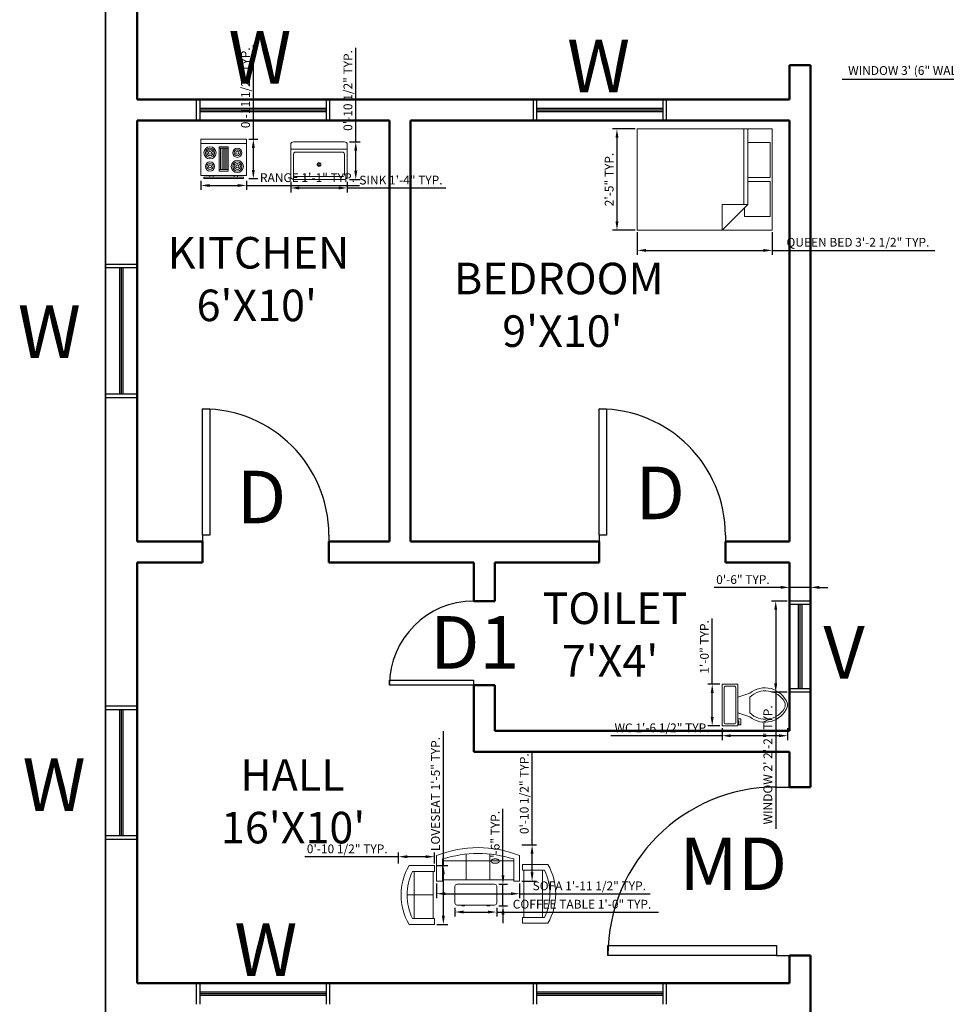
# Model space of a CAD drawing. Units: inches. Extents: x -25308 to -23933, y 10755 to 11996.
# Tile 2 of 6: x -25306 to -25042, y 11402 to 11683. Entities that reach past the tile are written whole.
import ezdxf

# ---------------------------------------------------------------- set-up
doc = ezdxf.new("R2010")
doc.units = ezdxf.units.IN
for name, color, linetype, lineweight in [('A-ANNO-DIMS', 2, 'Continuous', 18), ('A-ANNO-SYMB', 3, 'Continuous', 18), ('A-AREA-IDEN', 7, 'Continuous', 18), ('A-DOOR', 3, 'Continuous', 25), ('A-FLOR-FIXT', 8, 'Continuous', 18), ('A-FURN', 8, 'Continuous', 18), ('A-GLAZ', 4, 'Continuous', 25), ('A-WALL', 7, 'Continuous', 50), ('C-PROP', 30, 'Continuous', 35)]:
    doc.layers.add(name, color=color, linetype=linetype, lineweight=lineweight)
doc.styles.get("Standard").update_dxf_attribs({"font": 'arial.ttf'})
doc.dimstyles.new('ISO-25', dxfattribs={"dimtxt": 2.5, "dimasz": 2.5, "dimexe": 1.25, "dimexo": 0.625, "dimtad": 1, "dimdec": 0, "dimlunit": 3, "dimtxsty": 'Standard', "dimcen": 2.5, "dimadec": 0, "dimazin": 0, "dimtfac": 1, "dimtdec": 0, "dimtmove": 0, "dimatfit": 3, "dimfxl": 1, "dimarcsym": 0})

# ---------------------------------------------------------------- blocks, each defined once
blk = doc.blocks.new('*U8')
for p, q in [((0, 0), (0, -100)), ((750, 0), (750, -100))]:
    blk.add_line(p, q)
blk.add_lwpolyline([(0, 0), (0, 750), (43.75, 750), (43.75, 0)], close=True)
blk.add_arc((0, 0), 750, 0, 90)
blk = doc.blocks.new('Bed - Queen')
for p, q in [((0, -80.00003), (0, 0)), ((0, 0), (59.99999, 0)), ((59.99999, 0), (59.99999, -80.00003)), ((7.99999, -1.2), (28.79998, -1.2)), ((7.99999, -14.4), (7.99999, -1.2)), ((28.79998, -1.2), (28.79998, -14.4)), ((31.19999, -1.2), (51.99999, -1.2)), ((31.19999, -14.4), (31.19999, -1.2)), ((51.99999, -1.2), (51.99999, -16.4)), ((0, -14.4), (44.8, -14.4)), ((44.8, -16.8), (0, -16.8)), ((59.99999, -29.6), (44.8, -14.4)), ((44.8, -14.4), (44.8, -29.6)), ((51.99999, -16.4), (46.79936, -16.4)), ((44.8, -29.6), (59.99999, -29.6)), ((59.99999, -80.00003), (0, -80.00003))]:
    blk.add_line(p, q)
blk = doc.blocks.new('Range-Oven - 30 in top')
for p, q in [((0, -3), (30, -3)), ((12, -6), (18, -6)), ((13, -20), (13, -6)), ((14, -6), (14, -20)), ((15, -20), (15, -6)), ((16, -6), (16, -20)), ((17, -20), (17, -6)), ((6, -24), (6, -25)), ((8, -25), (8, -24)), ((18, -20), (12, -20)), ((22, -25), (22, -24)), ((24, -24), (24, -25))]:
    blk.add_line(p, q)
for points in [[(0, -24), (0, 0), (30, 0), (30, -24)], [(12, -21), (12, -5), (18, -5), (18, -21)], [(2, -26), (2, -25), (28, -25), (28, -26)]]:
    blk.add_lwpolyline(points, close=True)
for centre, radius in [((6, -9), 4), ((6, -9), 3), ((24, -9), 3), ((6, -9), 2), ((6, -9), 1), ((24, -9), 2), ((24, -9), 1), ((6, -18), 3), ((6, -18), 2), ((6, -18), 1), ((24, -18), 4), ((24, -18), 3), ((24, -18), 2), ((24, -18), 1)]:
    blk.add_circle(centre, radius)
blk = doc.blocks.new('Sink-single - 30 in top')
blk.add_line((-15, -3.999996), (15, -3.999996))
for points in [[(-13.5, 0), (13.5, 0)], [(-15, -18.499996), (-15, -1.5)], [(15, -1.5), (15, -18.499996)], [(-13.5, -17.499996), (-13.5, -6.499996)], [(-12.5, -5.499996), (12.5, -5.499996)], [(13.5, -6.499996), (13.5, -17.499996)], [(13.5, -19.999996), (-13.5, -19.999996)], [(12.5, -18.499996), (-12.5, -18.499996)]]:
    blk.add_lwpolyline(points)
for radius in [1, 0.5]:
    blk.add_circle((0, -11.999996), radius)
for centre, radius, start, end in [((-13.5, -1.5), 1.5, 90, 180), ((13.5, -1.5), 1.5, 0, 90), ((-12.5, -6.499996), 1, 90, 180), ((12.5, -6.499996), 1, 0, 90), ((-13.5, -18.499996), 1.5, 180, 270), ((-12.5, -17.499996), 1, 180, 270), ((12.5, -17.499996), 1, 270, 0), ((13.5, -18.499996), 1.5, 270, 0)]:
    blk.add_arc(centre, radius, start, end)
blk = doc.blocks.new('Toilet - top')
for p, q in [((9.5, -6), (9.5, -2)), ((-10, -8.5), (-8, -8.5)), ((-10, -9.5), (-10, -8.5)), ((-7, -9.5), (-10, -9.5)), ((-8, -8.5), (-8, -8)), ((-7, -8), (-7, -9.5)), ((-4, -8), (-6, -14)), ((4, -8), (6, -14)), ((4, -14), (-4, -14))]:
    blk.add_line(p, q)
blk.add_lwpolyline([(10.5, -8), (10.5, 0), (-10.5, 0), (-10.5, -8)], close=True)
for points in [[(-9.5, -2), (-9.5, -6)], [(8.5, -1), (-8.5, -1)], [(-8.5, -7), (8.5, -7)]]:
    blk.add_lwpolyline(points)
for centre, radius, start, end in [((-8.62, -1.88), 0.884, 81.8699, 188.1301), ((8.62, -1.88), 0.884, 351.8699, 98.1301), ((-8.62, -6.12), 0.884, 171.8699, 278.1301), ((8.62, -6.12), 0.884, 261.8699, 8.1301), ((3.52, -21.58), 12.17, 141.4691, 247.9714), ((4.2, -21.82), 11.33, 136.3677, 238.9468), ((-3.52, -21.58), 12.17, 292.0284, 38.5307), ((-4.2, -21.82), 11.33, 301.053, 43.6321), ((0, -27.88), 4, 245.7318, 294.2682), ((0, -29), 4, 254.8605, 285.1395)]:
    blk.add_arc(centre, radius, start, end)
blk = doc.blocks.new('Desk - 30 x 60 in.')
for p, q in [((-26.999995, 0), (26.999995, 0)), ((-29.999995, -27), (-29.999995, -3)), ((29.999995, -3), (29.999995, -27)), ((26.999995, -30), (-26.999995, -30)), ((-20.000005, -30), (-20.000005, -31)), ((-20.000005, -31), (-16.000005, -31)), ((-16.000005, -31), (-16.000005, -30)), ((15.999995, -31), (15.999995, -30)), ((19.999995, -31), (15.999995, -31)), ((19.999995, -30), (19.999995, -31))]:
    blk.add_line(p, q)
for centre, start, end in [((-26.499995, -3.5), 98.1301, 171.8699), ((26.499995, -3.5), 8.130102, 81.8699), ((-26.499995, -26.5), 188.1301, 261.8699), ((26.499995, -26.5), 278.1301, 351.8699)]:
    blk.add_arc(centre, 3.535534, start, end)
blk = doc.blocks.new('Sofa - Roundback 7 ft.')
for p, q in [((-12.00002, -32.4421), (-12.00003, -6.5971)), ((11.99997, -32.4421), (11.99998, -6.5971)), ((-36.000027, -34), (-36.000027, -11.4696)), ((-35.999844, -13.3819), (35.9998, -13.3819)), ((35.99998, -34), (35.99998, -11.4696)), ((-36.000027, -32.4421), (35.99998, -32.4421))]:
    blk.add_line(p, q)
for points in [[(-36.000027, -34), (-42.000027, -34), (-42.000027, -8)], [(41.99998, -8), (41.99998, -34), (35.99998, -34)]]:
    blk.add_lwpolyline(points)
for centre, radius, start, end in [((0, -114.25), 114.25, 68.43141, 111.5686), ((-0.00001, -127.1968), 121.1968, 72.72033, 107.2797)]:
    blk.add_arc(centre, radius, start, end)
blk = doc.blocks.new('Sofa - Roundback Loveseat 5 ft.')
for p, q in [((0, -32.44198), (0, -5.99998)), ((-24, -33.99998), (-24, -11.46958)), ((-23.9998, -13.38178), (23.99986, -13.38178)), ((24.00004, -33.99998), (24.00004, -11.46958)), ((-24, -32.44198), (24.00004, -32.44198))]:
    blk.add_line(p, q)
for points in [[(-24, -33.99998), (-30, -33.99998), (-30, -7.99998)], [(30.00004, -7.99998), (30.00004, -33.99998), (24.00004, -33.99998)]]:
    blk.add_lwpolyline(points)
for centre, radius, start, end in [((0, -60.24998), 60.24998, 60.13715, 119.8628), ((0, -61.38438), 55.38444, 64.32083, 115.6792)]:
    blk.add_arc(centre, radius, start, end)
blk = doc.blocks.new('WIN-36-9IN')
for p, q in [((0, 9), (0, 0)), ((1, 9), (1, 0)), ((37, 9), (37, 0)), ((38, 9), (38, 0)), ((1, 5), (37, 5)), ((1, 4.5), (37, 4.5)), ((1, 4), (37, 4))]:
    blk.add_line(p, q)
blk = doc.blocks.new('WIN-24-6IN')
for p, q in [((0, 26), (6, 26)), ((0, 25), (6, 25)), ((2.5, 1), (2.5, 25)), ((3, 1), (3, 25)), ((3.5, 1), (3.5, 25)), ((0, 1), (6, 1)), ((0, 0), (6, 0))]:
    blk.add_line(p, q)
blk = doc.blocks.new('WIN-36-6IN')
for p, q in [((0, 6), (0, 0)), ((1, 6), (1, 0)), ((37, 6), (37, 0)), ((38, 6), (38, 0)), ((1, 3.5), (37, 3.5)), ((1, 3), (37, 3)), ((1, 2.5), (37, 2.5))]:
    blk.add_line(p, q)
blk = doc.blocks.new('*D184')
at = {"layer": 'A-ANNO-DIMS', "color": 0, "lineweight": -2, "transparency": 16777216}
for p, q in [((-25015.44, 11660.75), (-25015.44, 11667.07)), ((-24977.44, 11660.75), (-24977.44, 11667.07)), ((-25015.44, 11665.82), (-25071.37, 11665.82)), ((-24979.94, 11665.82), (-25012.94, 11665.82))]:
    blk.add_line(p, q, dxfattribs=at)
at = {"layer": 'A-ANNO-DIMS', "color": 0, "transparency": 16777216}
for points in [[(-25012.94, 11666.24), (-25012.94, 11665.4), (-25015.44, 11665.82)], [(-24979.94, 11666.24), (-24979.94, 11665.4), (-24977.44, 11665.82)]]:
    blk.add_solid(points, dxfattribs=at)
at = {"layer": 'Defpoints', "color": 0, "transparency": 16777216}
for p in [(-25015.44, 11665.82), (-25015.44, 11660.12), (-24977.44, 11660.12)]:
    blk.add_point(p, dxfattribs=at)
at = {"layer": 'A-ANNO-DIMS', "color": 0, "transparency": 16777216, "insert": (-25044.66, 11668.09), "char_height": 2.5, "attachment_point": 5}
blk.add_mtext('WINDOW 3\' (6" WALL) 3\'-2" TYP.', dxfattribs=at)
blk = doc.blocks.new('*D186')
at = {"layer": 'A-ANNO-DIMS', "color": 0, "lineweight": -2, "transparency": 16777216}
for p, q in [((-25087.07, 11517.12), (-25091.59, 11517.12)), ((-25090.34, 11514.62), (-25090.34, 11493.62)), ((-25087.07, 11491.12), (-25091.59, 11491.12)), ((-25090.34, 11491.12), (-25090.34, 11452.16))]:
    blk.add_line(p, q, dxfattribs=at)
at = {"layer": 'A-ANNO-DIMS', "color": 0, "transparency": 16777216}
for points in [[(-25090.76, 11514.62), (-25089.93, 11514.62), (-25090.34, 11517.12)], [(-25090.76, 11493.62), (-25089.93, 11493.62), (-25090.34, 11491.12)]]:
    blk.add_solid(points, dxfattribs=at)
at = {"layer": 'Defpoints', "color": 0, "transparency": 16777216}
for p in [(-25086.44, 11517.12), (-25090.34, 11491.12), (-25086.44, 11491.12)]:
    blk.add_point(p, dxfattribs=at)
at = {"layer": 'A-ANNO-DIMS', "color": 0, "transparency": 16777216, "insert": (-25092.26, 11470.39), "char_height": 2.5, "attachment_point": 5, "rotation": 90}
blk.add_mtext('WINDOW 2\' 2\'-2" TYP.', dxfattribs=at)
blk = doc.blocks.new('*D187')
at = {"layer": 'A-ANNO-DIMS', "color": 0, "lineweight": -2, "transparency": 16777216}
for p, q in [((-25088.94, 11521.02), (-25107.93, 11521.02)), ((-25086.44, 11517.75), (-25086.44, 11522.27)), ((-25080.44, 11521.02), (-25086.44, 11521.02)), ((-25080.44, 11517.75), (-25080.44, 11522.27)), ((-25077.94, 11521.02), (-25075.44, 11521.02))]:
    blk.add_line(p, q, dxfattribs=at)
at = {"layer": 'A-ANNO-DIMS', "color": 0, "transparency": 16777216}
for points in [[(-25088.94, 11521.44), (-25088.94, 11520.6), (-25086.44, 11521.02)], [(-25077.94, 11521.44), (-25077.94, 11520.6), (-25080.44, 11521.02)]]:
    blk.add_solid(points, dxfattribs=at)
at = {"layer": 'Defpoints', "color": 0, "transparency": 16777216}
for p in [(-25086.44, 11521.02), (-25086.44, 11517.12), (-25080.44, 11517.12)]:
    blk.add_point(p, dxfattribs=at)
at = {"layer": 'A-ANNO-DIMS', "color": 0, "transparency": 16777216, "insert": (-25099.69, 11522.92), "char_height": 2.5, "attachment_point": 5}
blk.add_mtext('0\'-6" TYP.', dxfattribs=at)
blk = doc.blocks.new('*D192')
at = {"layer": 'A-ANNO-DIMS', "color": 0, "lineweight": -2, "transparency": 16777216}
for p, q in [((-25185.1, 11441.7), (-25185.1, 11479.98)), ((-25187, 11441.7), (-25183.85, 11441.7)), ((-25185.1, 11427.41), (-25185.1, 11439.2)), ((-25187, 11424.91), (-25183.85, 11424.91))]:
    blk.add_line(p, q, dxfattribs=at)
at = {"layer": 'A-ANNO-DIMS', "color": 0, "transparency": 16777216}
for points in [[(-25185.52, 11439.2), (-25184.68, 11439.2), (-25185.1, 11441.7)], [(-25185.52, 11427.41), (-25184.68, 11427.41), (-25185.1, 11424.91)]]:
    blk.add_solid(points, dxfattribs=at)
at = {"layer": 'Defpoints', "color": 0, "transparency": 16777216}
for p in [(-25187.62, 11441.7), (-25185.1, 11441.7), (-25187.62, 11424.91)]:
    blk.add_point(p, dxfattribs=at)
at = {"layer": 'A-ANNO-DIMS', "color": 0, "transparency": 16777216, "insert": (-25187.02, 11462.09), "char_height": 2.5, "attachment_point": 5, "rotation": 90}
blk.add_mtext('LOVESEAT 1\'-5" TYP.', dxfattribs=at)
blk = doc.blocks.new('*D193')
at = {"layer": 'A-ANNO-DIMS', "color": 0, "lineweight": -2, "transparency": 16777216}
for p, q in [((-25197.88, 11442.32), (-25197.88, 11445.46)), ((-25187.62, 11442.32), (-25187.62, 11445.46)), ((-25197.88, 11444.21), (-25224.64, 11444.21)), ((-25190.12, 11444.21), (-25195.38, 11444.21))]:
    blk.add_line(p, q, dxfattribs=at)
at = {"layer": 'A-ANNO-DIMS', "color": 0, "transparency": 16777216}
for points in [[(-25195.38, 11444.63), (-25195.38, 11443.8), (-25197.88, 11444.21)], [(-25190.12, 11444.63), (-25190.12, 11443.8), (-25187.62, 11444.21)]]:
    blk.add_solid(points, dxfattribs=at)
at = {"layer": 'Defpoints', "color": 0, "transparency": 16777216}
for p in [(-25197.88, 11444.21), (-25197.88, 11441.7), (-25187.62, 11441.7)]:
    blk.add_point(p, dxfattribs=at)
at = {"layer": 'A-ANNO-DIMS', "color": 0, "transparency": 16777216, "insert": (-25212.51, 11446.13), "char_height": 2.5, "attachment_point": 5}
blk.add_mtext('0\'-10 1/2" TYP.', dxfattribs=at)
blk = doc.blocks.new('*D198')
at = {"layer": 'A-ANNO-DIMS', "color": 0, "lineweight": -2, "transparency": 16777216}
for p, q in [((-25187.05, 11436.59), (-25187.05, 11432.41)), ((-25163.36, 11436.59), (-25163.36, 11432.41)), ((-25184.55, 11433.66), (-25165.86, 11433.66)), ((-25163.36, 11433.66), (-25126.13, 11433.66))]:
    blk.add_line(p, q, dxfattribs=at)
at = {"layer": 'A-ANNO-DIMS', "color": 0, "transparency": 16777216}
for points in [[(-25184.55, 11434.08), (-25184.55, 11433.24), (-25187.05, 11433.66)], [(-25165.86, 11434.08), (-25165.86, 11433.24), (-25163.36, 11433.66)]]:
    blk.add_solid(points, dxfattribs=at)
at = {"layer": 'Defpoints', "color": 0, "transparency": 16777216}
for p in [(-25187.05, 11437.21), (-25163.36, 11437.21), (-25163.36, 11433.66)]:
    blk.add_point(p, dxfattribs=at)
at = {"layer": 'A-ANNO-DIMS', "color": 0, "transparency": 16777216, "insert": (-25143.5, 11435.58), "char_height": 2.5, "attachment_point": 5}
blk.add_mtext('SOFA 1\'-11 1/2" TYP.', dxfattribs=at)
blk = doc.blocks.new('*D199')
at = {"layer": 'A-ANNO-DIMS', "color": 0, "lineweight": -2, "transparency": 16777216}
for p, q in [((-25159.81, 11447.56), (-25159.81, 11474.31)), ((-25162.73, 11447.56), (-25158.56, 11447.56)), ((-25159.81, 11439.71), (-25159.81, 11445.06)), ((-25162.73, 11437.21), (-25158.56, 11437.21))]:
    blk.add_line(p, q, dxfattribs=at)
at = {"layer": 'A-ANNO-DIMS', "color": 0, "transparency": 16777216}
for points in [[(-25160.22, 11445.06), (-25159.39, 11445.06), (-25159.81, 11447.56)], [(-25160.22, 11439.71), (-25159.39, 11439.71), (-25159.81, 11437.21)]]:
    blk.add_solid(points, dxfattribs=at)
at = {"layer": 'Defpoints', "color": 0, "transparency": 16777216}
for p in [(-25163.36, 11447.56), (-25159.81, 11447.56), (-25163.36, 11437.21)]:
    blk.add_point(p, dxfattribs=at)
at = {"layer": 'A-ANNO-DIMS', "color": 0, "transparency": 16777216, "insert": (-25161.72, 11462.18), "char_height": 2.5, "attachment_point": 5, "rotation": 90}
blk.add_mtext('0\'-10 1/2" TYP.', dxfattribs=at)
blk = doc.blocks.new('*D204')
at = {"layer": 'A-ANNO-DIMS', "color": 0, "lineweight": -2, "transparency": 16777216}
for p, q in [((-25181.83, 11429.6), (-25181.83, 11427.18)), ((-25179.33, 11428.43), (-25172.39, 11428.43)), ((-25169.89, 11429.6), (-25169.89, 11427.18)), ((-25169.89, 11428.43), (-25123.76, 11428.43))]:
    blk.add_line(p, q, dxfattribs=at)
at = {"layer": 'A-ANNO-DIMS', "color": 0, "transparency": 16777216}
for points in [[(-25179.33, 11428.85), (-25179.33, 11428.02), (-25181.83, 11428.43)], [(-25172.39, 11428.85), (-25172.39, 11428.02), (-25169.89, 11428.43)]]:
    blk.add_solid(points, dxfattribs=at)
at = {"layer": 'Defpoints', "color": 0, "transparency": 16777216}
for p in [(-25181.83, 11430.22), (-25169.89, 11430.22), (-25169.89, 11428.43)]:
    blk.add_point(p, dxfattribs=at)
at = {"layer": 'A-ANNO-DIMS', "color": 0, "transparency": 16777216, "insert": (-25145.57, 11430.35), "char_height": 2.5, "attachment_point": 5}
blk.add_mtext('COFFEE TABLE 1\'-0" TYP.', dxfattribs=at)
blk = doc.blocks.new('*D205')
at = {"layer": 'A-ANNO-DIMS', "color": 0, "lineweight": -2, "transparency": 16777216}
for p, q in [((-25168.1, 11438.89), (-25168.1, 11457.88)), ((-25169.26, 11436.39), (-25166.85, 11436.39)), ((-25168.1, 11430.22), (-25168.1, 11436.39)), ((-25169.26, 11430.22), (-25166.85, 11430.22)), ((-25168.1, 11427.72), (-25168.1, 11425.22))]:
    blk.add_line(p, q, dxfattribs=at)
at = {"layer": 'A-ANNO-DIMS', "color": 0, "transparency": 16777216}
for points in [[(-25168.51, 11438.89), (-25167.68, 11438.89), (-25168.1, 11436.39)], [(-25168.51, 11427.72), (-25167.68, 11427.72), (-25168.1, 11430.22)]]:
    blk.add_solid(points, dxfattribs=at)
at = {"layer": 'Defpoints', "color": 0, "transparency": 16777216}
for p in [(-25169.89, 11436.39), (-25168.1, 11436.39), (-25169.89, 11430.22)]:
    blk.add_point(p, dxfattribs=at)
at = {"layer": 'A-ANNO-DIMS', "color": 0, "transparency": 16777216, "insert": (-25170, 11449.64), "char_height": 2.5, "attachment_point": 5, "rotation": 90}
blk.add_mtext('0\'-6" TYP.', dxfattribs=at)
blk = doc.blocks.new('*D206')
at = {"layer": 'A-ANNO-DIMS', "color": 0, "lineweight": -2, "transparency": 16777216}
for p, q in [((-25129.83, 11622.27), (-25129.83, 11615.87)), ((-25091.33, 11622.27), (-25091.33, 11615.87)), ((-25127.33, 11617.12), (-25093.83, 11617.12)), ((-25091.33, 11617.12), (-25044.98, 11617.12))]:
    blk.add_line(p, q, dxfattribs=at)
at = {"layer": 'A-ANNO-DIMS', "color": 0, "transparency": 16777216}
for points in [[(-25127.33, 11617.53), (-25127.33, 11616.7), (-25129.83, 11617.12)], [(-25093.83, 11617.53), (-25093.83, 11616.7), (-25091.33, 11617.12)]]:
    blk.add_solid(points, dxfattribs=at)
at = {"layer": 'Defpoints', "color": 0, "transparency": 16777216}
for p in [(-25129.83, 11622.89), (-25091.33, 11622.89), (-25091.33, 11617.12)]:
    blk.add_point(p, dxfattribs=at)
at = {"layer": 'A-ANNO-DIMS', "color": 0, "transparency": 16777216, "insert": (-25066.91, 11619.11), "char_height": 2.5, "attachment_point": 5}
blk.add_mtext('QUEEN BED 3\'-2 1/2" TYP.', dxfattribs=at)
blk = doc.blocks.new('*D207')
at = {"layer": 'A-ANNO-DIMS', "color": 0, "lineweight": -2, "transparency": 16777216}
for p, q in [((-25130.46, 11651.77), (-25136.86, 11651.77)), ((-25135.61, 11649.27), (-25135.61, 11625.39)), ((-25130.46, 11622.89), (-25136.86, 11622.89))]:
    blk.add_line(p, q, dxfattribs=at)
at = {"layer": 'A-ANNO-DIMS', "color": 0, "transparency": 16777216}
for points in [[(-25136.02, 11649.27), (-25135.19, 11649.27), (-25135.61, 11651.77)], [(-25136.02, 11625.39), (-25135.19, 11625.39), (-25135.61, 11622.89)]]:
    blk.add_solid(points, dxfattribs=at)
at = {"layer": 'Defpoints', "color": 0, "transparency": 16777216}
for p in [(-25129.83, 11651.77), (-25135.61, 11622.89), (-25129.83, 11622.89)]:
    blk.add_point(p, dxfattribs=at)
at = {"layer": 'A-ANNO-DIMS', "color": 0, "transparency": 16777216, "insert": (-25137.51, 11637.33), "char_height": 2.5, "attachment_point": 5, "rotation": 90}
blk.add_mtext('2\'-5" TYP.', dxfattribs=at)
blk = doc.blocks.new('*D210')
at = {"layer": 'A-ANNO-DIMS', "color": 0, "lineweight": -2, "transparency": 16777216}
for p, q in [((-25254.24, 11636.95), (-25254.24, 11634.38)), ((-25241.22, 11636.95), (-25241.22, 11634.38)), ((-25251.74, 11635.63), (-25243.72, 11635.63)), ((-25241.22, 11635.63), (-25208.97, 11635.63))]:
    blk.add_line(p, q, dxfattribs=at)
at = {"layer": 'A-ANNO-DIMS', "color": 0, "transparency": 16777216}
for points in [[(-25251.74, 11636.04), (-25251.74, 11635.21), (-25254.24, 11635.63)], [(-25243.72, 11636.04), (-25243.72, 11635.21), (-25241.22, 11635.63)]]:
    blk.add_solid(points, dxfattribs=at)
at = {"layer": 'Defpoints', "color": 0, "transparency": 16777216}
for p in [(-25254.24, 11637.58), (-25241.22, 11637.58), (-25241.22, 11635.63)]:
    blk.add_point(p, dxfattribs=at)
at = {"layer": 'A-ANNO-DIMS', "color": 0, "transparency": 16777216, "insert": (-25223.85, 11637.54), "char_height": 2.5, "attachment_point": 5}
blk.add_mtext('RANGE 1\'-1" TYP.', dxfattribs=at)
blk = doc.blocks.new('*D211')
at = {"layer": 'A-ANNO-DIMS', "color": 0, "lineweight": -2, "transparency": 16777216}
for p, q in [((-25239.27, 11648.86), (-25239.27, 11675.61)), ((-25240.6, 11648.86), (-25238.02, 11648.86)), ((-25239.27, 11640.08), (-25239.27, 11646.36)), ((-25240.6, 11637.58), (-25238.02, 11637.58))]:
    blk.add_line(p, q, dxfattribs=at)
at = {"layer": 'A-ANNO-DIMS', "color": 0, "transparency": 16777216}
for points in [[(-25239.69, 11646.36), (-25238.85, 11646.36), (-25239.27, 11648.86)], [(-25239.69, 11640.08), (-25238.85, 11640.08), (-25239.27, 11637.58)]]:
    blk.add_solid(points, dxfattribs=at)
at = {"layer": 'Defpoints', "color": 0, "transparency": 16777216}
for p in [(-25241.22, 11648.86), (-25239.27, 11648.86), (-25241.22, 11637.58)]:
    blk.add_point(p, dxfattribs=at)
at = {"layer": 'A-ANNO-DIMS', "color": 0, "transparency": 16777216, "insert": (-25241.19, 11663.49), "char_height": 2.5, "attachment_point": 5, "rotation": 90}
blk.add_mtext('0\'-11 1/2" TYP.', dxfattribs=at)
blk = doc.blocks.new('*D212')
at = {"layer": 'A-ANNO-DIMS', "color": 0, "lineweight": -2, "transparency": 16777216}
for p, q in [((-25105.65, 11478.72), (-25137.36, 11478.72)), ((-25105.65, 11480.9), (-25105.65, 11477.47)), ((-25089.45, 11478.72), (-25103.15, 11478.72)), ((-25086.95, 11480.9), (-25086.95, 11477.47))]:
    blk.add_line(p, q, dxfattribs=at)
at = {"layer": 'A-ANNO-DIMS', "color": 0, "transparency": 16777216}
for points in [[(-25103.15, 11479.14), (-25103.15, 11478.3), (-25105.65, 11478.72)], [(-25089.45, 11479.14), (-25089.45, 11478.3), (-25086.95, 11478.72)]]:
    blk.add_solid(points, dxfattribs=at)
at = {"layer": 'Defpoints', "color": 0, "transparency": 16777216}
for p in [(-25105.65, 11481.52), (-25086.95, 11481.52), (-25105.65, 11478.72)]:
    blk.add_point(p, dxfattribs=at)
at = {"layer": 'A-ANNO-DIMS', "color": 0, "transparency": 16777216, "insert": (-25122.76, 11480.64), "char_height": 2.5, "attachment_point": 5}
blk.add_mtext('WC 1\'-6 1/2" TYP.', dxfattribs=at)
blk = doc.blocks.new('*D213')
at = {"layer": 'A-ANNO-DIMS', "color": 0, "lineweight": -2, "transparency": 16777216}
for p, q in [((-25108.46, 11493.41), (-25108.46, 11512.16)), ((-25106.28, 11493.41), (-25109.71, 11493.41)), ((-25108.46, 11484.02), (-25108.46, 11490.91)), ((-25106.28, 11481.52), (-25109.71, 11481.52))]:
    blk.add_line(p, q, dxfattribs=at)
at = {"layer": 'A-ANNO-DIMS', "color": 0, "transparency": 16777216}
for points in [[(-25108.87, 11490.91), (-25108.04, 11490.91), (-25108.46, 11493.41)], [(-25108.87, 11484.02), (-25108.04, 11484.02), (-25108.46, 11481.52)]]:
    blk.add_solid(points, dxfattribs=at)
at = {"layer": 'Defpoints', "color": 0, "transparency": 16777216}
for p in [(-25108.46, 11493.41), (-25105.65, 11493.41), (-25105.65, 11481.52)]:
    blk.add_point(p, dxfattribs=at)
at = {"layer": 'A-ANNO-DIMS', "color": 0, "transparency": 16777216, "insert": (-25110.36, 11504.04), "char_height": 2.5, "attachment_point": 5, "rotation": 90}
blk.add_mtext('1\'-0" TYP.', dxfattribs=at)
blk = doc.blocks.new('*D216')
at = {"layer": 'A-ANNO-DIMS', "color": 0, "lineweight": -2, "transparency": 16777216}
for p, q in [((-25228.62, 11636.71), (-25228.62, 11633.67)), ((-25212.49, 11636.71), (-25212.49, 11633.67)), ((-25226.12, 11634.92), (-25214.99, 11634.92)), ((-25212.49, 11634.92), (-25184.4, 11634.92))]:
    blk.add_line(p, q, dxfattribs=at)
at = {"layer": 'A-ANNO-DIMS', "color": 0, "transparency": 16777216}
for points in [[(-25226.12, 11635.34), (-25226.12, 11634.5), (-25228.62, 11634.92)], [(-25214.99, 11635.34), (-25214.99, 11634.5), (-25212.49, 11634.92)]]:
    blk.add_solid(points, dxfattribs=at)
at = {"layer": 'Defpoints', "color": 0, "transparency": 16777216}
for p in [(-25228.62, 11637.34), (-25212.49, 11637.34), (-25212.49, 11634.92)]:
    blk.add_point(p, dxfattribs=at)
at = {"layer": 'A-ANNO-DIMS', "color": 0, "transparency": 16777216, "insert": (-25197.19, 11636.84), "char_height": 2.5, "attachment_point": 5}
blk.add_mtext('SINK 1\'-4" TYP.', dxfattribs=at)
blk = doc.blocks.new('*D217')
at = {"layer": 'A-ANNO-DIMS', "color": 0, "lineweight": -2, "transparency": 16777216}
for p, q in [((-25210.08, 11648.09), (-25210.08, 11674.84)), ((-25211.87, 11648.09), (-25208.83, 11648.09)), ((-25210.08, 11639.84), (-25210.08, 11645.59)), ((-25211.87, 11637.34), (-25208.83, 11637.34))]:
    blk.add_line(p, q, dxfattribs=at)
at = {"layer": 'A-ANNO-DIMS', "color": 0, "transparency": 16777216}
for points in [[(-25210.49, 11645.59), (-25209.66, 11645.59), (-25210.08, 11648.09)], [(-25210.49, 11639.84), (-25209.66, 11639.84), (-25210.08, 11637.34)]]:
    blk.add_solid(points, dxfattribs=at)
at = {"layer": 'Defpoints', "color": 0, "transparency": 16777216}
for p in [(-25212.49, 11648.09), (-25210.08, 11648.09), (-25212.49, 11637.34)]:
    blk.add_point(p, dxfattribs=at)
at = {"layer": 'A-ANNO-DIMS', "color": 0, "transparency": 16777216, "insert": (-25211.99, 11662.72), "char_height": 2.5, "attachment_point": 5, "rotation": 90}
blk.add_mtext('0\'-10 1/2" TYP.', dxfattribs=at)

msp = doc.modelspace()

# ---------------------------------------------------------------- linework, layer by layer
at = {"layer": 'A-WALL'}
for p, q in [((-25272.44, 11660.12), (-25272.44, 11780.12)), ((-25086.44, 11660.12), (-25086.44, 11669.94)), ((-25086.44, 11669.94), (-25080.44, 11669.94)), ((-25080.44, 11464.06), (-25080.44, 11669.94)), ((-25272.44, 11660.12), (-25086.44, 11660.12)), ((-25272.44, 11654.12), (-25200.44, 11654.12)), ((-25272.44, 11534.12), (-25272.44, 11654.12)), ((-25200.44, 11534.12), (-25200.44, 11654.12)), ((-25194.44, 11534.12), (-25194.44, 11654.12)), ((-25194.44, 11654.12), (-25086.44, 11654.12)), ((-25086.44, 11534.12), (-25086.44, 11654.12)), ((-25272.44, 11534.12), (-25253.74, 11534.12)), ((-25253.74, 11534.12), (-25253.74, 11528.12)), ((-25217.74, 11534.12), (-25217.74, 11528.12)), ((-25217.74, 11534.12), (-25200.44, 11534.12)), ((-25194.44, 11534.12), (-25140.68, 11534.12)), ((-25140.68, 11534.12), (-25140.68, 11528.12)), ((-25104.68, 11534.12), (-25104.68, 11528.12)), ((-25104.68, 11534.12), (-25086.44, 11534.12)), ((-25272.44, 11528.12), (-25253.74, 11528.12)), ((-25272.44, 11408.12), (-25272.44, 11528.12)), ((-25217.74, 11528.12), (-25176.44, 11528.12)), ((-25176.44, 11517.12), (-25176.44, 11528.12)), ((-25176.44, 11517.12), (-25176.44, 11528.12)), ((-25176.44, 11517.12), (-25176.44, 11528.12)), ((-25170.44, 11528.12), (-25140.68, 11528.12)), ((-25170.44, 11517.12), (-25170.44, 11528.12)), ((-25170.44, 11517.12), (-25170.44, 11528.12)), ((-25170.44, 11517.12), (-25170.44, 11528.12)), ((-25104.68, 11528.12), (-25086.44, 11528.12)), ((-25086.44, 11480.12), (-25086.44, 11528.12)), ((-25176.44, 11517.12), (-25170.44, 11517.12)), ((-25176.44, 11474.12), (-25176.44, 11493.12)), ((-25176.44, 11474.12), (-25176.44, 11493.12)), ((-25176.44, 11474.12), (-25176.44, 11493.12)), ((-25176.44, 11493.12), (-25170.44, 11493.12)), ((-25170.44, 11480.12), (-25170.44, 11493.12)), ((-25170.44, 11480.12), (-25170.44, 11493.12)), ((-25170.44, 11480.12), (-25170.44, 11493.12)), ((-25170.44, 11480.12), (-25086.44, 11480.12)), ((-25176.44, 11474.12), (-25086.44, 11474.12)), ((-25086.44, 11464.06), (-25086.44, 11474.12)), ((-25086.44, 11464.06), (-25080.44, 11464.06)), ((-25086.44, 11408.12), (-25086.44, 11416.06)), ((-25086.44, 11416.06), (-25080.44, 11416.06)), ((-25080.44, 11213.16), (-25080.44, 11416.06)), ((-25272.44, 11408.12), (-25086.44, 11408.12))]:
    msp.add_line(p, q, dxfattribs=at)
at = {"layer": 'C-PROP'}
msp.add_line((-25281.44, 10811.12), (-25281.44, 11915.12), dxfattribs=at)

# ---------------------------------------------------------------- block references
at = {"layer": 'A-DOOR', "xscale": 0.0480000000000013, "yscale": 0.0480000000000013, "zscale": 0.0480000000000013}
for p in [(-25253.74, 11535.92), (-25140.68, 11535.92)]:
    msp.add_blockref('*U8', p, dxfattribs=at)
at = {"layer": 'A-DOOR', "rotation": 90}
for p, xscale, yscale, zscale in [((-25176.47, 11493.12), 0.0320000000000009, 0.0320000000000009, 0.0320000000000009), ((-25090.14, 11416.06), 0.0640305237838995, 0.0640305237838995, 0.0640305237838995)]:
    msp.add_blockref('*U8', p, dxfattribs=dict(at, xscale=xscale, yscale=yscale, zscale=zscale))
at = {"layer": 'A-FLOR-FIXT'}
for name, p, xscale, yscale, zscale in [('Range-Oven - 30 in top', (-25254.24, 11648.86), 0.4338097128947254, 0.4338097128947254, 0.4338097128947254), ('Sink-single - 30 in top', (-25220.56, 11648.09), 0.5374838416175965, 0.5374838416175965, 0.5374838416175965)]:
    msp.add_blockref(name, p, dxfattribs=dict(at, xscale=xscale, yscale=yscale, zscale=zscale))
at = {"layer": 'A-FLOR-FIXT', "xscale": 0.5659332238665749, "yscale": 0.5659332238665749, "zscale": 0.5659332238665749, "rotation": 90}
msp.add_blockref('Toilet - top', (-25105.65, 11487.47), dxfattribs=at)
at = {"layer": 'A-FURN'}
for name, p, xscale, yscale, zscale, rotation in [('Bed - Queen', (-25091.33, 11651.77), 0.4812808282186369, 0.4812808282186369, 0.4812808282186369, 270), ('Sofa - Roundback Loveseat 5 ft.', (-25197.13, 11433.3), 0.2798473955820579, 0.2798473955820579, 0.2798473955820579, 89.99999999999999), ('Sofa - Roundback Loveseat 5 ft.', (-25153.06, 11433.63), 0.2798473955820579, 0.2798473955820579, 0.2798473955820579, 270)]:
    msp.add_blockref(name, p, dxfattribs=dict(at, xscale=xscale, yscale=yscale, zscale=zscale, rotation=rotation))
for name, p, xscale, yscale, zscale in [('Sofa - Roundback 7 ft.', (-25175.2, 11446.8), 0.2820316080914415, 0.2820316080914415, 0.2820316080914415), ('Desk - 30 x 60 in.', (-25175.86, 11436.39), 0.1990306524997052, 0.1990306524997052, 0.1990306524997052)]:
    msp.add_blockref(name, p, dxfattribs=dict(at, xscale=xscale, yscale=yscale, zscale=zscale))
at = {"layer": 'A-GLAZ'}
for name, p, rotation in [('WIN-36-6IN', (-25217.44, 11660.12), 180), ('WIN-36-6IN', (-25121.44, 11660.12), 180), ('WIN-36-9IN', (-25281.44, 11613.12), 270.0000000000198), ('WIN-24-6IN', (-25080.44, 11517.12), 180), ('WIN-36-9IN', (-25281.44, 11487.12), 270.0000000000303), ('WIN-36-6IN', (-25217.44, 11408.12), 180), ('WIN-36-6IN', (-25121.44, 11408.12), 180)]:
    msp.add_blockref(name, p, dxfattribs=dict(at, rotation=rotation))

# ---------------------------------------------------------------- texts
at = {"layer": 'A-ANNO-SYMB', "char_height": 15, "attachment_point": 1}
for s, insert in [('{W}', (-25246.39, 11679.71)), ('{W}', (-25149.82, 11677.21)), ('{W}', (-25306.42, 11601.44)), ('{D}', (-25130.3, 11555.47)), ('{D}', (-25243.97, 11554.28)), ('{D1}', (-25188.88, 11512.82)), ('{V}', (-25076.75, 11510)), ('{W}', (-25305.06, 11472.25)), ('{MD}', (-25117.79, 11449.68)), ('{W}', (-25244.7, 11425.21))]:
    msp.add_mtext_dynamic_manual_height_columns(s, width=1123.2502, gutter_width=12.5, heights=[0], dxfattribs=dict(at, insert=insert))
at = {"layer": 'A-AREA-IDEN', "char_height": 9, "attachment_point": 1}
for s, insert in [("{KITCHEN\\P   6'X10'}", (-25263.7, 11620.94)), ("{BEDROOM\\P     9'X10'}", (-25182.06, 11613.6)), ("{TOILET\\P  7'X4'}", (-25156.83, 11519.56)), ("{   HALL\\P 16'X10'}", (-25251.24, 11472.01))]:
    msp.add_mtext_dynamic_manual_height_columns(s, width=1489.8169, gutter_width=12.5, heights=[0], dxfattribs=dict(at, insert=insert))

# ---------------------------------------------------------------- dimensions: what is measured, and where the dimension line sits
at = {"layer": 'A-ANNO-DIMS'}
for base, p1, p2, angle, text, picture, middle in [((-25015.44, 11665.82), (-24977.44, 11660.12), (-25015.44, 11660.12), 180, 'WINDOW 3\' (6" WALL) <> TYP.', '*D184', (-25044.66, 11668.09)), ((-25239.27, 11648.86), (-25241.22, 11637.58), (-25241.22, 11648.86), 90, '<> TYP.', '*D211', (-25241.19, 11663.49)), ((-25210.0755, 11648.0877), (-25212.4942, 11637.338), (-25212.4942, 11648.0877), 90, '<> TYP.', '*D217', (-25211.9932, 11662.716)), ((-25135.61, 11622.89), (-25129.83, 11651.77), (-25129.83, 11622.89), 270, '<> TYP.', '*D207', (-25137.51, 11637.33)), ((-25086.44, 11521.02), (-25080.44, 11517.12), (-25086.44, 11517.12), 180, '<> TYP.', '*D187', (-25099.69, 11522.92)), ((-25090.34, 11491.12), (-25086.44, 11517.12), (-25086.44, 11491.12), 270, "WINDOW 2' <> TYP.", '*D186', (-25092.26, 11470.39)), ((-25108.46, 11493.41), (-25105.65, 11481.52), (-25105.65, 11493.41), 90, '<> TYP.', '*D213', (-25110.36, 11504.04)), ((-25105.65, 11478.72), (-25086.95, 11481.52), (-25105.65, 11481.52), 180, 'WC <> TYP.', '*D212', (-25122.76, 11480.64)), ((-25185.1, 11441.7), (-25187.62, 11424.91), (-25187.62, 11441.7), 90, 'LOVESEAT <> TYP.', '*D192', (-25187.02, 11462.09)), ((-25159.8051, 11447.5551), (-25163.3587, 11437.214), (-25163.3587, 11447.5551), 90, '<> TYP.', '*D199', (-25161.7228, 11462.1834)), ((-25168.1, 11436.39), (-25169.89, 11430.22), (-25169.89, 11436.39), 90, '<> TYP.', '*D205', (-25170, 11449.64)), ((-25197.88, 11444.21), (-25187.62, 11441.7), (-25197.88, 11441.7), 180, '<> TYP.', '*D193', (-25212.51, 11446.13))]:
    dim = msp.add_linear_dim(base=base, p1=p1, p2=p2, angle=angle, text=text, dimstyle='ISO-25', override={"dimdec": 1, "dimlfac": 1, "dimrnd": 0, "dimzin": 1, "dimdsep": 46, "dimlunit": 4, "dimfrac": 2}, dxfattribs=at)
    dim.commit()
    dim.dimension.update_dxf_attribs({"geometry": picture, "text_midpoint": middle})
for base, p1, p2, text, picture, middle in [((-25241.22, 11635.63), (-25254.24, 11637.58), (-25241.22, 11637.58), 'RANGE <> TYP.', '*D210', (-25223.85, 11637.54)), ((-25212.49, 11634.92), (-25228.62, 11637.34), (-25212.49, 11637.34), 'SINK <> TYP.', '*D216', (-25197.19, 11636.84)), ((-25091.33, 11617.12), (-25129.83, 11622.89), (-25091.33, 11622.89), 'QUEEN BED <> TYP.', '*D206', (-25066.91, 11619.11)), ((-25163.36, 11433.66), (-25187.05, 11437.21), (-25163.36, 11437.21), 'SOFA <> TYP.', '*D198', (-25143.5, 11435.58)), ((-25169.89, 11428.43), (-25181.83, 11430.22), (-25169.89, 11430.22), 'COFFEE TABLE <> TYP.', '*D204', (-25145.57, 11430.35))]:
    dim = msp.add_linear_dim(base=base, p1=p1, p2=p2, text=text, dimstyle='ISO-25', override={"dimdec": 1, "dimlfac": 1, "dimrnd": 0, "dimzin": 1, "dimdsep": 46, "dimlunit": 4, "dimfrac": 2}, dxfattribs=at)
    dim.commit()
    dim.dimension.update_dxf_attribs({"geometry": picture, "text_midpoint": middle})

doc.saveas('drawing.dxf')
